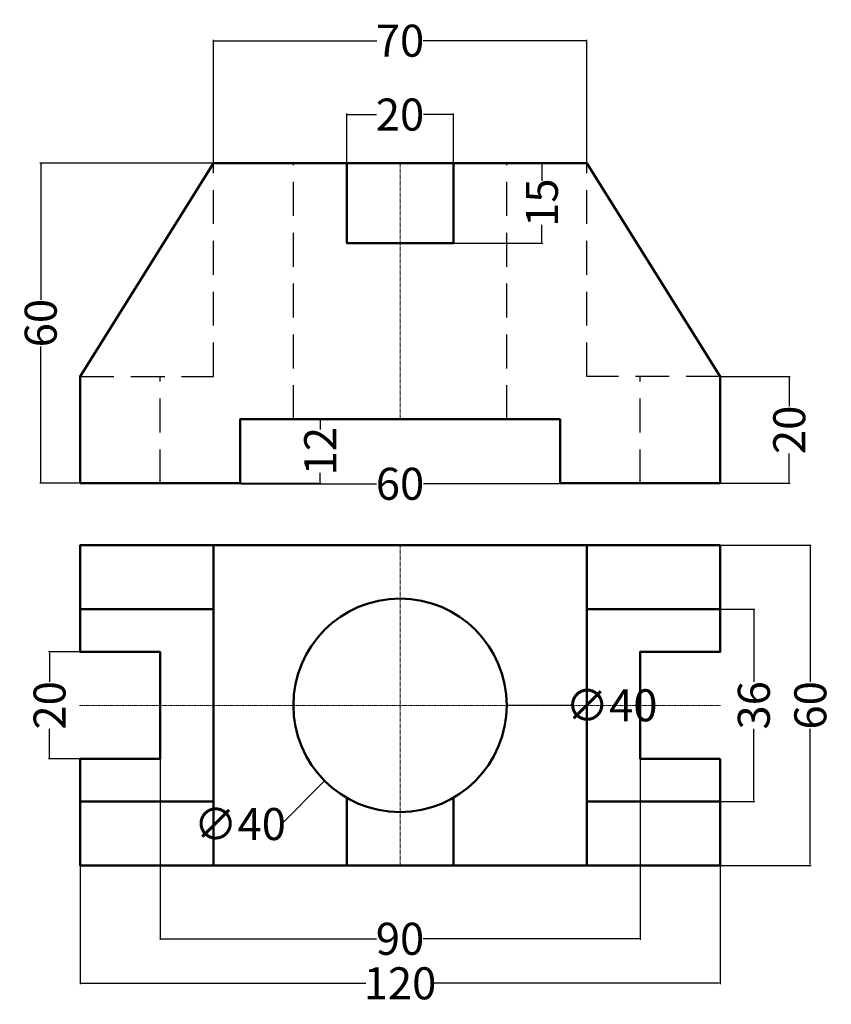
# Model space of a CAD drawing. Units: millimetres. Extents: x 11 to 163, y 4 to 188.
import ezdxf

# ---------------------------------------------------------------- set-up
doc = ezdxf.new("R2010")
doc.units = ezdxf.units.MM
doc.header["$MEASUREMENT"] = 0
doc.linetypes.add('CENTER2', pattern=[1.125, 0.75, -0.125, 0.125, -0.125])
doc.linetypes.add('HIDDEN', pattern=[9.525, 6.35, -3.175])
for name, color, linetype, lineweight in [('M-CNTR', 4, 'CENTER2', 18), ('M-CONS', 8, 'Continuous', 13), ('M-DIMS', 2, 'Continuous', 25), ('M-HIDN', 3, 'HIDDEN', 25), ('M-OUTL', 7, 'Continuous', 50)]:
    doc.layers.add(name, color=color, linetype=linetype, lineweight=lineweight)
doc.styles.get("Standard").update_dxf_attribs({"font": 'arial.ttf'})
doc.dimstyles.get("Standard").update_dxf_attribs({"dimtxt": 6, "dimasz": 0.18, "dimexe": 0.18, "dimexo": 0.0625, "dimgap": 0.09, "dimtad": 0, "dimtoh": 1, "dimdec": 0, "dimzin": 0, "dimdsep": 46, "dimtxsty": 'Standard', "dimcen": 0.09, "dimadec": 0, "dimazin": 0, "dimtfac": 1, "dimtdec": 0, "dimtofl": 0, "dimtmove": 0, "dimatfit": 3, "dimfxl": 1, "dimtolj": 1, "dimtzin": 0, "dimarcsym": 0})

# ---------------------------------------------------------------- blocks, each defined once
blk = doc.blocks.new('*D1')
at = {"layer": 'Defpoints', "color": 0, "transparency": 16777216}
for p in [(116.87, 184.56), (46.87, 161.64), (116.87, 161.64)]:
    blk.add_point(p, dxfattribs=at)
at = {"layer": 'M-DIMS', "color": 0, "lineweight": -2, "transparency": 16777216}
for p, q in [((46.87, 161.7), (46.87, 184.74)), ((47.05, 184.56), (77.51, 184.56)), ((116.69, 184.56), (86.22, 184.56)), ((116.87, 161.7), (116.87, 184.74))]:
    blk.add_line(p, q, dxfattribs=at)
at = {"layer": 'M-DIMS', "color": 0, "transparency": 16777216}
for points in [[(47.05, 184.59), (47.05, 184.53), (46.87, 184.56)], [(116.69, 184.59), (116.69, 184.53), (116.87, 184.56)]]:
    blk.add_solid(points, dxfattribs=at)
at = {"layer": 'M-DIMS', "color": 0, "transparency": 16777216, "insert": (81.87, 184.56), "char_height": 6, "attachment_point": 5}
blk.add_mtext('\\A1;70', dxfattribs=at)
blk = doc.blocks.new('*D2')
at = {"layer": 'Defpoints', "color": 0, "transparency": 16777216}
for p in [(91.87, 170.72), (71.87, 161.76), (91.87, 161.64)]:
    blk.add_point(p, dxfattribs=at)
at = {"layer": 'M-DIMS', "color": 0, "lineweight": -2, "transparency": 16777216}
for p, q in [((71.87, 161.82), (71.87, 170.9)), ((72.05, 170.72), (77.44, 170.72)), ((91.69, 170.72), (86.3, 170.72)), ((91.87, 161.7), (91.87, 170.9))]:
    blk.add_line(p, q, dxfattribs=at)
at = {"layer": 'M-DIMS', "color": 0, "transparency": 16777216}
for points in [[(72.05, 170.75), (72.05, 170.69), (71.87, 170.72)], [(91.69, 170.75), (91.69, 170.69), (91.87, 170.72)]]:
    blk.add_solid(points, dxfattribs=at)
at = {"layer": 'M-DIMS', "color": 0, "transparency": 16777216, "insert": (81.87, 170.72), "char_height": 6, "attachment_point": 5}
blk.add_mtext('\\A1;20', dxfattribs=at)
blk = doc.blocks.new('*D3')
at = {"layer": 'Defpoints', "color": 0, "transparency": 16777216}
for p in [(51.87, 113.64), (51.87, 101.64), (66.9, 101.64)]:
    blk.add_point(p, dxfattribs=at)
at = {"layer": 'M-DIMS', "color": 0, "lineweight": -2, "transparency": 16777216}
for p, q in [((51.93, 113.64), (67.08, 113.64)), ((66.9, 113.46), (66.9, 111.71)), ((66.9, 101.82), (66.9, 103.56)), ((51.93, 101.64), (67.08, 101.64))]:
    blk.add_line(p, q, dxfattribs=at)
at = {"layer": 'M-DIMS', "color": 0, "transparency": 16777216}
for points in [[(66.87, 113.46), (66.93, 113.46), (66.9, 113.64)], [(66.87, 101.82), (66.93, 101.82), (66.9, 101.64)]]:
    blk.add_solid(points, dxfattribs=at)
at = {"layer": 'M-DIMS', "color": 0, "transparency": 16777216, "insert": (66.9, 107.64), "char_height": 6, "attachment_point": 5, "rotation": 90}
blk.add_mtext('\\A1;12', dxfattribs=at)
blk = doc.blocks.new('*D4')
at = {"layer": 'Defpoints', "color": 0, "transparency": 16777216}
for p in [(91.87, 161.76), (91.87, 146.64), (108.47, 146.64)]:
    blk.add_point(p, dxfattribs=at)
at = {"layer": 'M-DIMS', "color": 0, "lineweight": -2, "transparency": 16777216}
for p, q in [((91.93, 161.76), (108.65, 161.76)), ((108.47, 161.58), (108.47, 158.33)), ((108.47, 146.82), (108.47, 150.07)), ((91.93, 146.64), (108.65, 146.64))]:
    blk.add_line(p, q, dxfattribs=at)
at = {"layer": 'M-DIMS', "color": 0, "transparency": 16777216}
for points in [[(108.44, 161.58), (108.5, 161.58), (108.47, 161.76)], [(108.44, 146.82), (108.5, 146.82), (108.47, 146.64)]]:
    blk.add_solid(points, dxfattribs=at)
at = {"layer": 'M-DIMS', "color": 0, "transparency": 16777216, "insert": (108.47, 154.2), "char_height": 6, "attachment_point": 5, "rotation": 90}
blk.add_mtext('\\A1;15', dxfattribs=at)
blk = doc.blocks.new('*D5')
at = {"layer": 'Defpoints', "color": 0, "transparency": 16777216}
for p in [(141.87, 121.64), (141.87, 101.64), (154.85, 101.64)]:
    blk.add_point(p, dxfattribs=at)
at = {"layer": 'M-DIMS', "color": 0, "lineweight": -2, "transparency": 16777216}
for p, q in [((141.93, 121.64), (155.03, 121.64)), ((154.85, 121.46), (154.85, 116.07)), ((154.85, 101.82), (154.85, 107.21)), ((141.93, 101.64), (155.03, 101.64))]:
    blk.add_line(p, q, dxfattribs=at)
at = {"layer": 'M-DIMS', "color": 0, "transparency": 16777216}
for points in [[(154.82, 121.46), (154.88, 121.46), (154.85, 121.64)], [(154.82, 101.82), (154.88, 101.82), (154.85, 101.64)]]:
    blk.add_solid(points, dxfattribs=at)
at = {"layer": 'M-DIMS', "color": 0, "transparency": 16777216, "insert": (154.85, 111.64), "char_height": 6, "attachment_point": 5, "rotation": 90}
blk.add_mtext('\\A1;20', dxfattribs=at)
blk = doc.blocks.new('*D6')
at = {"layer": 'Defpoints', "color": 0, "transparency": 16777216}
for p in [(51.87, 101.54), (111.87, 101.54), (111.87, 101.54)]:
    blk.add_point(p, dxfattribs=at)
at = {"layer": 'M-DIMS', "color": 0, "lineweight": -2, "transparency": 16777216}
for p, q in [((51.87, 101.61), (51.87, 101.72)), ((52.05, 101.54), (77.47, 101.54)), ((111.69, 101.54), (86.26, 101.54)), ((111.87, 101.61), (111.87, 101.72))]:
    blk.add_line(p, q, dxfattribs=at)
at = {"layer": 'M-DIMS', "color": 0, "transparency": 16777216}
for points in [[(52.05, 101.57), (52.05, 101.51), (51.87, 101.54)], [(111.69, 101.57), (111.69, 101.51), (111.87, 101.54)]]:
    blk.add_solid(points, dxfattribs=at)
at = {"layer": 'M-DIMS', "color": 0, "transparency": 16777216, "insert": (81.87, 101.54), "char_height": 6, "attachment_point": 5}
blk.add_mtext('\\A1;60', dxfattribs=at)
blk = doc.blocks.new('*D7')
at = {"layer": 'Defpoints', "color": 0, "transparency": 16777216}
for p in [(46.87, 161.64), (14.5, 101.64), (21.87, 101.64)]:
    blk.add_point(p, dxfattribs=at)
at = {"layer": 'M-DIMS', "color": 0, "lineweight": -2, "transparency": 16777216}
for p, q in [((46.81, 161.64), (14.32, 161.64)), ((14.5, 161.46), (14.5, 136.03)), ((14.5, 101.82), (14.5, 127.25)), ((21.81, 101.64), (14.32, 101.64))]:
    blk.add_line(p, q, dxfattribs=at)
at = {"layer": 'M-DIMS', "color": 0, "transparency": 16777216}
for points in [[(14.47, 161.46), (14.53, 161.46), (14.5, 161.64)], [(14.47, 101.82), (14.53, 101.82), (14.5, 101.64)]]:
    blk.add_solid(points, dxfattribs=at)
at = {"layer": 'M-DIMS', "color": 0, "transparency": 16777216, "insert": (14.5, 131.64), "char_height": 6, "attachment_point": 5, "rotation": 90}
blk.add_mtext('\\A1;60', dxfattribs=at)
blk = doc.blocks.new('*D8')
at = {"layer": 'Defpoints', "color": 0, "transparency": 16777216}
for p in [(95.99, 74.18), (67.74, 45.87)]:
    blk.add_point(p, dxfattribs=at)
at = {"layer": 'M-DIMS', "color": 0, "lineweight": -2, "transparency": 16777216}
for p, q in [((81.78, 60.02), (81.96, 60.02)), ((81.87, 59.93), (81.87, 60.11)), ((59.67, 37.78), (67.61, 45.74)), ((59.49, 37.78), (59.67, 37.78))]:
    blk.add_line(p, q, dxfattribs=at)
at = {"layer": 'M-DIMS', "color": 0, "transparency": 16777216}
blk.add_solid([(67.59, 45.76), (67.64, 45.72), (67.74, 45.87)], dxfattribs=at)
at = {"layer": 'M-DIMS', "color": 0, "transparency": 16777216, "insert": (51.85, 37.78), "char_height": 6, "attachment_point": 5}
blk.add_mtext('\\A1;∅40', dxfattribs=at)
blk = doc.blocks.new('*D9')
at = {"layer": 'Defpoints', "color": 0, "transparency": 16777216}
for p in [(21.87, 70.02), (16.16, 50.02), (21.87, 50.02)]:
    blk.add_point(p, dxfattribs=at)
at = {"layer": 'M-DIMS', "color": 0, "lineweight": -2, "transparency": 16777216}
for p, q in [((21.81, 70.02), (15.98, 70.02)), ((16.16, 69.84), (16.16, 64.45)), ((16.16, 50.2), (16.16, 55.6)), ((21.81, 50.02), (15.98, 50.02))]:
    blk.add_line(p, q, dxfattribs=at)
at = {"layer": 'M-DIMS', "color": 0, "transparency": 16777216}
for points in [[(16.13, 69.84), (16.19, 69.84), (16.16, 70.02)], [(16.13, 50.2), (16.19, 50.2), (16.16, 50.02)]]:
    blk.add_solid(points, dxfattribs=at)
at = {"layer": 'M-DIMS', "color": 0, "transparency": 16777216, "insert": (16.16, 60.02), "char_height": 6, "attachment_point": 5, "rotation": 90}
blk.add_mtext('\\A1;20', dxfattribs=at)
blk = doc.blocks.new('*D10')
at = {"layer": 'Defpoints', "color": 0, "transparency": 16777216}
for p in [(141.87, 78.02), (141.87, 42.02), (148.21, 42.02)]:
    blk.add_point(p, dxfattribs=at)
at = {"layer": 'M-DIMS', "color": 0, "lineweight": -2, "transparency": 16777216}
for p, q in [((141.93, 78.02), (148.39, 78.02)), ((148.21, 77.84), (148.21, 64.41)), ((148.21, 42.2), (148.21, 55.64)), ((141.93, 42.02), (148.39, 42.02))]:
    blk.add_line(p, q, dxfattribs=at)
at = {"layer": 'M-DIMS', "color": 0, "transparency": 16777216}
for points in [[(148.18, 77.84), (148.24, 77.84), (148.21, 78.02)], [(148.18, 42.2), (148.24, 42.2), (148.21, 42.02)]]:
    blk.add_solid(points, dxfattribs=at)
at = {"layer": 'M-DIMS', "color": 0, "transparency": 16777216, "insert": (148.21, 60.02), "char_height": 6, "attachment_point": 5, "rotation": 90}
blk.add_mtext('\\A1;36', dxfattribs=at)
blk = doc.blocks.new('*D11')
at = {"layer": 'Defpoints', "color": 0, "transparency": 16777216}
for p in [(141.87, 90.02), (141.87, 30.02), (158.8, 30.02)]:
    blk.add_point(p, dxfattribs=at)
at = {"layer": 'M-DIMS', "color": 0, "lineweight": -2, "transparency": 16777216}
for p, q in [((141.93, 90.02), (158.98, 90.02)), ((158.8, 89.84), (158.8, 64.42)), ((158.8, 30.2), (158.8, 55.63)), ((141.93, 30.02), (158.98, 30.02))]:
    blk.add_line(p, q, dxfattribs=at)
at = {"layer": 'M-DIMS', "color": 0, "transparency": 16777216}
for points in [[(158.77, 89.84), (158.83, 89.84), (158.8, 90.02)], [(158.77, 30.2), (158.83, 30.2), (158.8, 30.02)]]:
    blk.add_solid(points, dxfattribs=at)
at = {"layer": 'M-DIMS', "color": 0, "transparency": 16777216, "insert": (158.8, 60.02), "char_height": 6, "attachment_point": 5, "rotation": 90}
blk.add_mtext('\\A1;60', dxfattribs=at)
blk = doc.blocks.new('*D12')
at = {"layer": 'Defpoints', "color": 0, "transparency": 16777216}
for p in [(36.87, 50.02), (126.87, 50.02), (126.87, 16.28)]:
    blk.add_point(p, dxfattribs=at)
at = {"layer": 'M-DIMS', "color": 0, "lineweight": -2, "transparency": 16777216}
for p, q in [((36.87, 49.96), (36.87, 16.1)), ((126.87, 49.96), (126.87, 16.1)), ((37.05, 16.28), (77.49, 16.28)), ((126.69, 16.28), (86.24, 16.28))]:
    blk.add_line(p, q, dxfattribs=at)
at = {"layer": 'M-DIMS', "color": 0, "transparency": 16777216}
for points in [[(37.05, 16.31), (37.05, 16.25), (36.87, 16.28)], [(126.69, 16.31), (126.69, 16.25), (126.87, 16.28)]]:
    blk.add_solid(points, dxfattribs=at)
at = {"layer": 'M-DIMS', "color": 0, "transparency": 16777216, "insert": (81.87, 16.28), "char_height": 6, "attachment_point": 5}
blk.add_mtext('\\A1;90', dxfattribs=at)
blk = doc.blocks.new('*D13')
at = {"layer": 'Defpoints', "color": 0, "transparency": 16777216}
for p in [(21.87, 30.02), (141.87, 30.02), (141.87, 7.94)]:
    blk.add_point(p, dxfattribs=at)
at = {"layer": 'M-DIMS', "color": 0, "lineweight": -2, "transparency": 16777216}
for p, q in [((21.87, 29.96), (21.87, 7.76)), ((141.87, 29.96), (141.87, 7.76)), ((22.05, 7.94), (75.44, 7.94)), ((141.69, 7.94), (88.29, 7.94))]:
    blk.add_line(p, q, dxfattribs=at)
at = {"layer": 'M-DIMS', "color": 0, "transparency": 16777216}
for points in [[(22.05, 7.97), (22.05, 7.91), (21.87, 7.94)], [(141.69, 7.97), (141.69, 7.91), (141.87, 7.94)]]:
    blk.add_solid(points, dxfattribs=at)
at = {"layer": 'M-DIMS', "color": 0, "transparency": 16777216, "insert": (81.87, 7.94), "char_height": 6, "attachment_point": 5}
blk.add_mtext('\\A1;120', dxfattribs=at)
blk = doc.blocks.new('*D14')
at = {"layer": 'Defpoints', "color": 0, "transparency": 16777216}
for p in [(61.87, 60.02), (101.87, 60.02)]:
    blk.add_point(p, dxfattribs=at)
at = {"layer": 'M-DIMS', "color": 0, "lineweight": -2, "transparency": 16777216}
for p, q in [((81.78, 60.02), (81.96, 60.02)), ((81.87, 59.93), (81.87, 60.11)), ((113.87, 60.03), (102.05, 60.02))]:
    blk.add_line(p, q, dxfattribs=at)
at = {"layer": 'M-DIMS', "color": 0, "transparency": 16777216}
blk.add_solid([(102.05, 60.06), (102.05, 60), (101.87, 60.02)], dxfattribs=at)
at = {"layer": 'M-DIMS', "color": 0, "transparency": 16777216, "insert": (121.51, 60.03), "char_height": 6, "attachment_point": 5}
blk.add_mtext('\\A1;∅40', dxfattribs=at)

msp = doc.modelspace()

# ---------------------------------------------------------------- linework, layer by layer
at = {"layer": 'M-CNTR'}
for p, q in [((81.87, 113.64), (81.87, 161.76)), ((81.87, 29.9), (81.87, 90.14)), ((21.75, 60.02), (141.99, 60.02))]:
    msp.add_line(p, q, dxfattribs=at)
at = {"layer": 'M-CONS'}
for p, q in [((36.87, 90.02), (36.87, 90.14)), ((126.87, 90.02), (126.87, 90.14)), ((36.87, 29.9), (36.87, 30.02)), ((126.87, 29.9), (126.87, 30.02))]:
    msp.add_line(p, q, dxfattribs=at)
at = {"layer": 'M-HIDN'}
for p, q in [((61.87, 113.64), (61.87, 161.64)), ((101.87, 113.64), (101.87, 161.64)), ((36.87, 101.64), (36.87, 121.64)), ((126.87, 101.64), (126.87, 121.64))]:
    msp.add_line(p, q, dxfattribs=at)
for points in [[(21.87, 121.64), (46.87, 121.64), (46.87, 161.64)], [(141.87, 121.64), (116.87, 121.64), (116.87, 161.64)]]:
    msp.add_lwpolyline(points, dxfattribs=at)
at = {"layer": 'M-OUTL'}
for p, q in [((46.87, 29.9), (46.87, 90.14)), ((116.87, 29.9), (116.87, 90.14)), ((21.87, 78.02), (46.87, 78.02)), ((116.87, 78.02), (141.87, 78.02)), ((71.87, 29.9), (71.87, 42.7)), ((91.87, 29.9), (91.87, 42.7)), ((21.87, 42.02), (46.87, 42.02)), ((116.87, 42.02), (141.87, 42.02))]:
    msp.add_line(p, q, dxfattribs=at)
for points in [[(21.87, 101.64), (21.87, 121.64), (46.87, 161.64), (116.87, 161.64), (141.87, 121.64), (141.87, 101.64), (111.87, 101.64), (111.87, 113.64), (51.87, 113.64), (51.87, 101.64)], [(141.87, 50.02), (141.87, 30.02), (21.87, 30.02), (21.87, 50.02), (36.87, 50.02), (36.87, 70.02), (21.87, 70.02), (21.87, 90.02), (141.87, 90.02), (141.87, 70.02), (126.87, 70.02), (126.87, 50.02)]]:
    msp.add_lwpolyline(points, close=True, dxfattribs=at)
msp.add_lwpolyline([(91.87, 161.76), (91.87, 146.64), (71.87, 146.64), (71.87, 161.76)], dxfattribs=at)
msp.add_circle((81.87, 60.02), 20, dxfattribs=at)

# ---------------------------------------------------------------- dimensions: what is measured, and where the dimension line sits
at = {"layer": 'M-DIMS'}
for base, p1, p2, picture, middle in [((116.87, 184.56), (46.87, 161.64), (116.87, 161.64), '*D1', (81.87, 184.56)), ((91.87, 170.72), (71.87, 161.76), (91.87, 161.64), '*D2', (81.87, 170.72)), ((111.87, 101.54), (51.87, 101.54), (111.87, 101.54), '*D6', (81.87, 101.54)), ((126.87, 16.28), (36.87, 50.02), (126.87, 50.02), '*D12', (81.87, 16.28)), ((141.87, 7.94), (21.87, 30.02), (141.87, 30.02), '*D13', (81.87, 7.94))]:
    dim = msp.add_linear_dim(base=base, p1=p1, p2=p2, dimstyle='Standard', override={"dimclrd": 0, "dimclre": 0, "dimclrt": 0}, dxfattribs=at)
    dim.commit()
    dim.dimension.update_dxf_attribs({"geometry": picture, "text_midpoint": middle})
for base, p1, p2, picture, middle in [((14.5, 101.64), (46.87, 161.64), (21.87, 101.64), '*D7', (14.5, 131.64)), ((108.47, 146.64), (91.87, 161.76), (91.87, 146.64), '*D4', (108.47, 154.2)), ((154.85, 101.64), (141.87, 121.64), (141.87, 101.64), '*D5', (154.85, 111.64)), ((66.9, 101.64), (51.87, 113.64), (51.87, 101.64), '*D3', (66.9, 107.64)), ((158.8, 30.02), (141.87, 90.02), (141.87, 30.02), '*D11', (158.8, 60.02)), ((148.21, 42.02), (141.87, 78.02), (141.87, 42.02), '*D10', (148.21, 60.02)), ((16.16, 50.02), (21.87, 70.02), (21.87, 50.02), '*D9', (16.16, 60.02))]:
    dim = msp.add_linear_dim(base=base, p1=p1, p2=p2, angle=90, dimstyle='Standard', override={"dimclrd": 0, "dimclre": 0, "dimclrt": 0}, dxfattribs=at)
    dim.commit()
    dim.dimension.update_dxf_attribs({"geometry": picture, "text_midpoint": middle})
for p1, p2, override, picture, middle in [((95.99, 74.18), (67.74, 45.87), {"dimclrd": 0, "dimclre": 0, "dimclrt": 0}, '*D8', (51.85, 37.78)), ((61.87, 60.02), (101.87, 60.02), {"dimdec": 0, "dimlfac": 1, "dimrnd": 0, "dimzin": 0, "dimdsep": 46, "dimlunit": 2}, '*D14', (113.87, 60.03))]:
    dim = msp.add_diameter_dim_2p(p1=p1, p2=p2, dimstyle='Standard', override=override, dxfattribs=at)
    dim.commit()
    dim.dimension.update_dxf_attribs({"geometry": picture, "text_midpoint": middle, "dimtype": 163})

doc.saveas('drawing.dxf')
